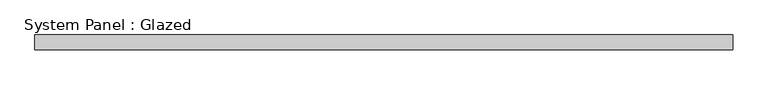
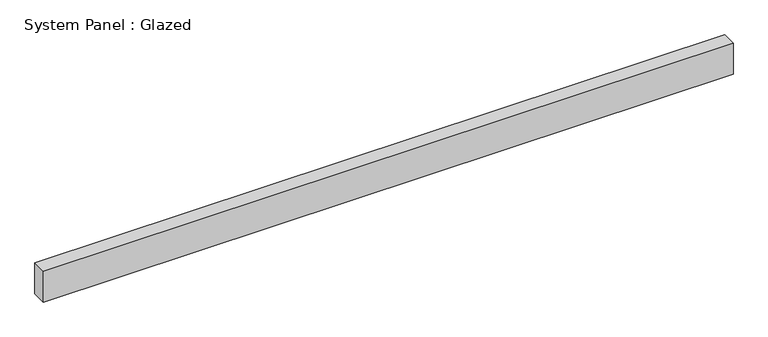
"""IFC4 building model written with IfcOpenShell, lengths in millimetres: plate geometry, System Panel : Glazed."""

from ifc_helpers import new_model, si_unit, origin, origin_with_axes, place, context, project, spatial, polyline, outline, extrude, source, transform, mapped, element, save


def system_panel_glazed_4956db27(model_context):
    return source(origin(), model_context, "Body", "SweptSolid", [
        extrude(outline(polyline([(603.2499999, 19.05), (-603.2499999, 19.05), (-603.2499999, 44.45), (603.2499999, 44.45), (603.2499999, 19.05)])), origin_with_axes(), (0.0, 0.0, 1.0), 57.15),
    ])


if __name__ == "__main__":
    model = new_model("IFC4")
    model_context = context("Model", 3, world=origin())
    ifc_project = project(units=[si_unit("LENGTHUNIT", "METRE", prefix="MILLI")], contexts=[model_context])
    site = spatial("IfcSite", under=ifc_project)
    building = spatial("IfcBuilding", under=site)
    placement = place(None, origin())
    system_panel_glazed_shape = system_panel_glazed_4956db27(model_context)
    element("IfcPlate", 1, ObjectType="System Panel : Glazed", at=placement, inside=building, context=model_context, shape_type="MappedRepresentation", body=[
        mapped(system_panel_glazed_shape, transform((0.0, 0.0, 0.0), x_axis=(1.0, 0.0, 0.0), y_axis=(0.0, 1.0, 0.0), z_axis=(0.0, 0.0, 1.0))),
    ])
    save(model, "model.ifc")

# Revit data of these elements
# Type "System Panel : Glazed"
#   Construction Type Id = "GSP4R"
#   Analytic Construction = "1/8 in Pilkington single glazing"
#   Visual Light Transmittance = 0.9
#   Solar Heat Gain Coefficient = 0.86
#   Heat Transfer Coefficient (U) = 1.18115 BTU/(h·ft²·°F)
#   Define Thermal Properties by = 1
# Element 1 (IfcPlate, "System Panel : Glazed")
#   Materials on its faces: "Glass"
# Materials
#   "Glass": class "Glass", colour RGB 0 128 192, transparency 0.75, Description = "Soda Lime Glass", Cost = 0
